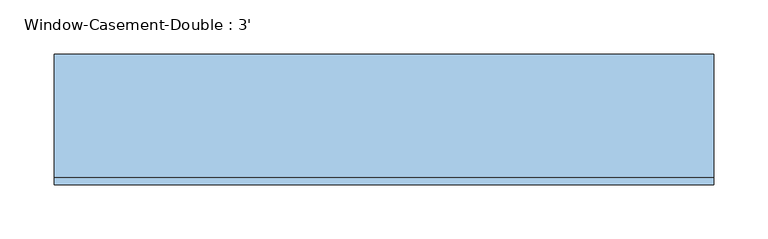
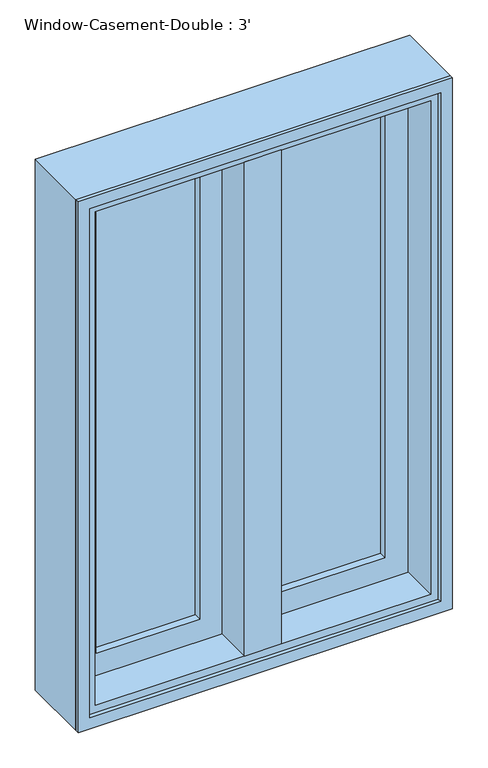
"""IFC4 building model written with IfcOpenShell, lengths in millimetres: window geometry, Window-Casement-Double : 3'."""

from ifc_helpers import new_model, si_unit, frame, origin, place, context, project, spatial, polyline, outline, extrude, faceted_brep, source, transform, mapped, element, save


def window_casement_double_3_e50e525e(model_context):
    return source(origin(), model_context, "Body", "SolidModel", [
        faceted_brep([(9.525, 69.85, 1816.1), (-9.525, 69.85, 1816.1), (-9.525, 19.05, 1816.1), (9.525, 19.05, 1816.1), (9.525, 69.85, 927.1), (9.525, 19.05, 927.1), (-9.525, 19.05, 927.1), (-9.525, 69.85, 927.1), (-9.525, 19.05, 946.15), (-9.525, 19.05, 1797.05), (-30.1625, 19.05, 946.15), (-30.1625, 19.05, 1797.05), (-30.1625, -44.45, 946.15), (-30.1625, -44.45, 1797.05), (30.1625, -44.45, 946.15), (30.1625, -44.45, 1797.05), (30.1625, 19.05, 946.15), (30.1625, 19.05, 1797.05), (9.525, 19.05, 946.15), (9.525, 19.05, 1797.05)], [[[0, 1, 2, 3]], [[4, 5, 6, 7]], [[1, 0, 4, 7]], [[2, 1, 7, 6, 8, 9]], [[9, 8, 10, 11]], [[11, 10, 12, 13]], [[13, 12, 14, 15]], [[15, 14, 16, 17]], [[17, 16, 18, 19]], [[0, 3, 19, 18, 5, 4]], [[18, 8, 6, 5]], [[9, 19, 3, 2]], [[8, 18, 16, 14, 12, 10]], [[19, 9, 11, 13, 15, 17]]]),
        extrude(outline(polyline([(-66.675, 50.8), (-66.675, 44.45), (-234.95, 44.45), (-234.95, 50.8), (-66.675, 50.8)])), frame((0.0, 0.0, 984.25), z_axis=(0.0, 0.0, 1.0), x_axis=(1.0, 0.0, 0.0)), (0.0, 0.0, 1.0), 774.7),
        extrude(outline(polyline([(-234.95, 31.75), (-234.95, 38.1), (-66.675, 38.1), (-66.675, 31.75), (-234.95, 31.75)])), frame((0.0, 0.0, 984.25), z_axis=(0.0, 0.0, 1.0), x_axis=(1.0, 0.0, 0.0)), (0.0, 0.0, 1.0), 774.7),
        extrude(outline(polyline([(234.95, 50.8), (234.95, 44.45), (66.675, 44.45), (66.675, 50.8), (234.95, 50.8)])), frame((0.0, 0.0, 984.25), z_axis=(0.0, 0.0, 1.0), x_axis=(1.0, 0.0, 0.0)), (0.0, 0.0, 1.0), 774.7),
        extrude(outline(polyline([(66.675, 31.75), (66.675, 38.1), (234.95, 38.1), (234.95, 31.75), (66.675, 31.75)])), frame((0.0, 0.0, 984.25), z_axis=(0.0, 0.0, 1.0), x_axis=(1.0, 0.0, 0.0)), (0.0, 0.0, 1.0), 774.7),
        extrude(outline(polyline([(1816.1, -292.1), (927.1, -292.1), (927.1, -9.525), (1816.1, -9.525), (1816.1, -292.1)]), holes=[polyline([(1758.95, -66.675), (984.25, -66.675), (984.25, -234.95), (1758.95, -234.95), (1758.95, -66.675)])]), frame((0.0, 19.05, 0.0), z_axis=(0.0, 1.0, 0.0), x_axis=(0.0, 0.0, 1.0)), (0.0, 0.0, 1.0), 44.45),
        extrude(outline(polyline([(927.1, 292.1), (1816.1, 292.1), (1816.1, 9.525), (927.1, 9.525), (927.1, 292.1)]), holes=[polyline([(984.25, 66.675), (1758.95, 66.675), (1758.95, 234.95), (984.25, 234.95), (984.25, 66.675)])]), frame((0.0, 19.05, 0.0), z_axis=(0.0, 1.0, 0.0), x_axis=(0.0, 0.0, 1.0)), (0.0, 0.0, 1.0), 44.45),
        extrude(outline(polyline([(1828.8, -304.8), (914.4, -304.8), (914.4, 304.8), (1828.8, 304.8), (1828.8, -304.8)]), holes=[polyline([(1809.75, 285.75), (933.45, 285.75), (933.45, -285.75), (1809.75, -285.75), (1809.75, 285.75)])]), frame((0.0, -50.8, 0.0), z_axis=(0.0, 1.0, 0.0), x_axis=(0.0, 0.0, 1.0)), (0.0, 0.0, 1.0), 6.35),
        faceted_brep([(273.05, 19.05, 1797.05), (273.05, -44.45, 1797.05), (-273.05, -44.45, 1797.05), (-273.05, 19.05, 1797.05), (292.1, 69.85, 1816.1), (292.1, 19.05, 1816.1), (-292.1, 19.05, 1816.1), (-292.1, 69.85, 1816.1), (304.8, -44.45, 1828.8), (304.8, 69.85, 1828.8), (-304.8, 69.85, 1828.8), (-304.8, -44.45, 1828.8), (-273.05, -44.45, 946.15), (-273.05, 19.05, 946.15), (-292.1, 19.05, 927.1), (-292.1, 69.85, 927.1), (-304.8, 69.85, 914.4), (-304.8, -44.45, 914.4), (273.05, -44.45, 946.15), (273.05, 19.05, 946.15), (292.1, 19.05, 927.1), (292.1, 69.85, 927.1), (304.8, 69.85, 914.4), (304.8, -44.45, 914.4)], [[[0, 1, 2, 3]], [[4, 5, 6, 7]], [[8, 9, 10, 11]], [[3, 2, 12, 13]], [[7, 6, 14, 15]], [[11, 10, 16, 17]], [[13, 12, 18, 19]], [[15, 14, 20, 21]], [[17, 16, 22, 23]], [[11, 17, 23, 8], [1, 18, 12, 2]], [[19, 18, 1, 0]], [[5, 20, 14, 6], [3, 13, 19, 0]], [[21, 20, 5, 4]], [[23, 22, 9, 8]], [[9, 22, 16, 10], [7, 15, 21, 4]]]),
    ])


if __name__ == "__main__":
    model = new_model("IFC4")
    model_context = context("Model", 3, world=origin())
    ifc_project = project(units=[si_unit("LENGTHUNIT", "METRE", prefix="MILLI")], contexts=[model_context])
    site = spatial("IfcSite", under=ifc_project)
    building = spatial("IfcBuilding", under=site)
    placement = place(None, origin())
    window_casement_double_3_shape = window_casement_double_3_e50e525e(model_context)
    element("IfcWindow", 1, ObjectType="Window-Casement-Double : 3'", at=placement, inside=building, context=model_context, shape_type="MappedRepresentation", body=[
        mapped(window_casement_double_3_shape, transform((0.0, 0.0, 0.0), x_axis=(1.0, 0.0, 0.0), y_axis=(0.0, 1.0, 0.0), z_axis=(0.0, 0.0, 1.0))),
    ])
    save(model, "model.ifc")

# Revit data of these elements
# Type "Window-Casement-Double : 3'"
#   Type Mark = "19"
#   Fire Rating = "0.5h"
#   Assembly Code = "B2020100"
#   Analytic Construction = "Double glazing - domestic"
#   Frame Extension [instance default] = 0' - 0 1/4"
#   Window Inset [instance default] = 0' - 0"
#   Wall Thickness [instance default] = 0' - 6"
#   Interior Wall Closure [instance default] = 0' - 2 1/4"
#   Half Width = 1' - 0"
#   Visual Light Transmittance = 0.81
#   Thermal Resistance (R) = 1.8146 (h·ft²·°F)/BTU
#   Solar Heat Gain Coefficient = 0.76
#   Rough Width = 2' - 0 1/2"
#   Rough Height = 3' - 0 1/2"
#   Height = 3' - 0"
#   Heat Transfer Coefficient (U) = 0.5511 BTU/(h·ft²·°F)
#   Exterior Wall Closure [instance default] = 0' - 1 1/4"
#   Extension Jamb [instance default] = 0' - 2 1/4"
#   Default Sill Height = 3' - 0"
#   Width = 2' - 0"
#   Muntin Visibility = yes
#   Interior Trim Visibility [instance default] = yes
#   Exterior Trim Visibility [instance default] = yes
#   Extension Jamb Visibility [instance default] = yes
#   Interior Trim Material = Wood - Stained
#   Muntin Pattern = Muntin Pattern_2x2 : Muntin Pattern_2x2
#   Interior Trim = Trim-Window-Interior-Flat : Picture Frame
#   Interior Frame Material = Wood - Stained
#   Glass Panel Material = Glass
#   Exterior Trim Material = Clad - White
#   Exterior Trim = Trim-Window-Exterior-Flat : with Sill
#   Exterior Frame Material = Clad - White
#   Wall Closure = (empty or 0)
# Element 1 (IfcWindow, "Window-Casement-Double : 3'")
#   Wall Thickness = 0' - 4"
#   Extension Jamb = 0' - 0 1/4"
#   Materials on its faces: "Wood - Stained", "Glass", "Clad - White"
# Materials
#   "Wood - Stained": class "Wood", colour RGB 224 178 126, transparency 0, Cost = 0
#   "Glass": class "Glass", colour RGB 0 128 192, transparency 0.75, Description = "Soda Lime Glass", Cost = 0
#   "Clad - White": class "Wood", colour RGB 242 242 238, transparency 0, Cost = 0
